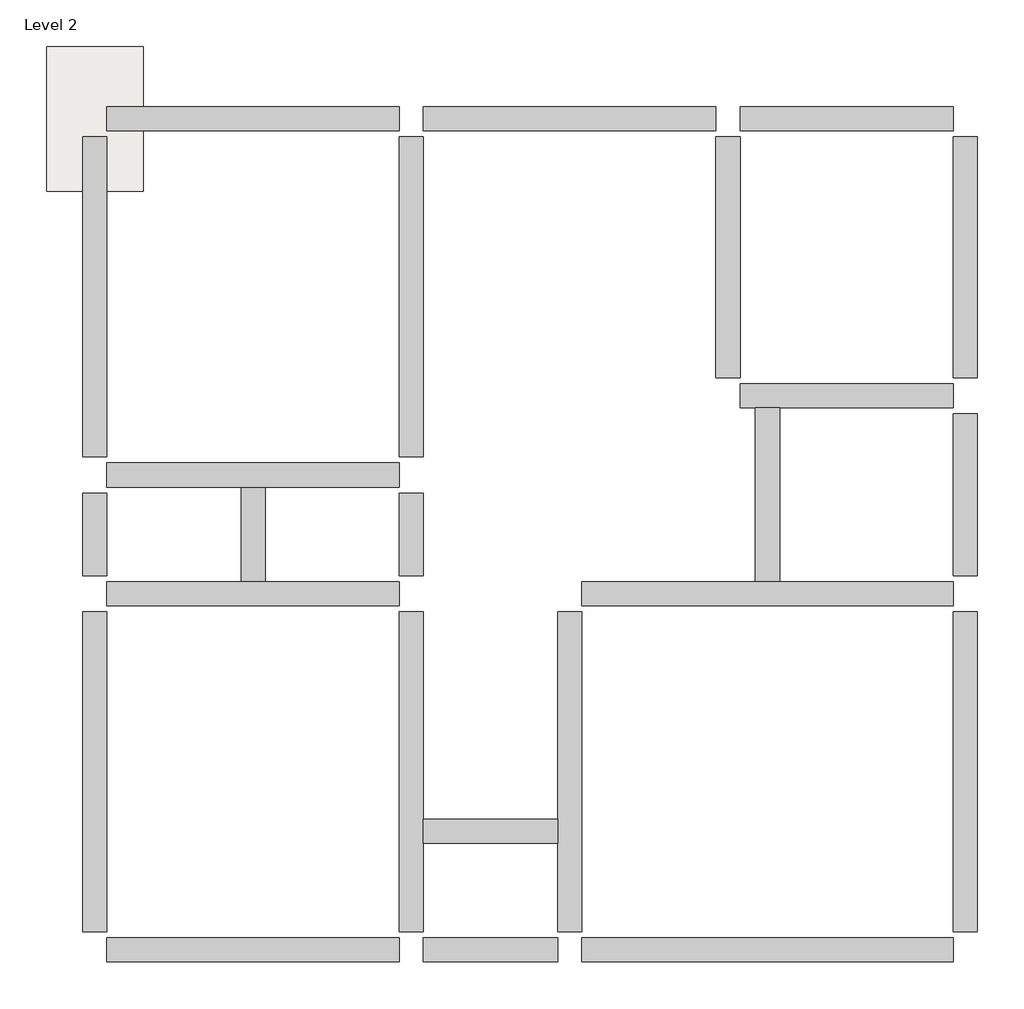
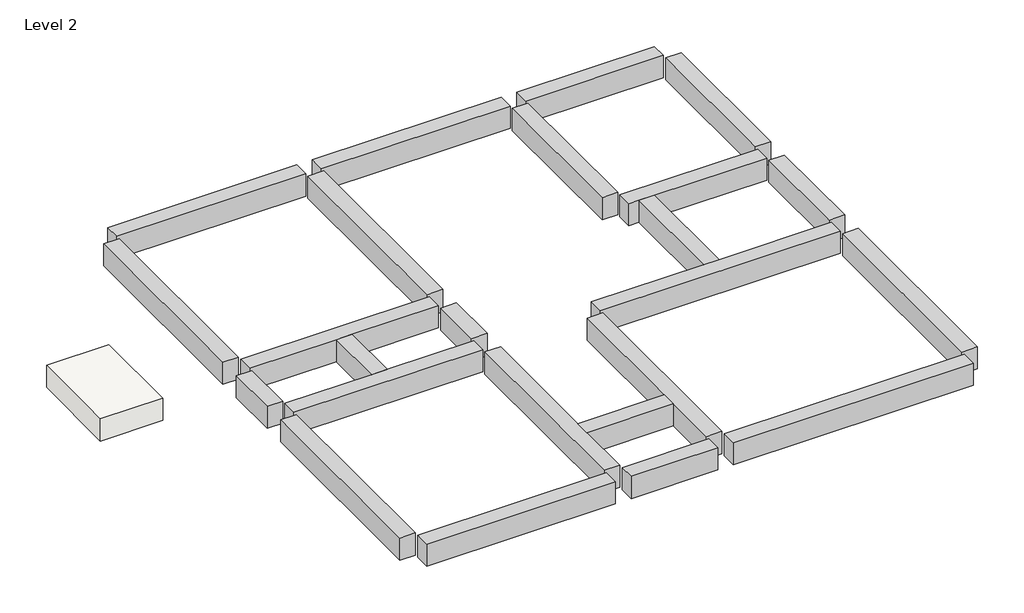
# One storey, part 1 of 5: 14 beams, 1 slab.
"""IFC4 building model written with IfcOpenShell, lengths in millimetres."""

from ifc_helpers import new_model, si_unit, frame, origin, place, context, project, spatial, polyline, outline, extrude, faceted_brep, element, save

model = new_model("IFC4")

# Units and contexts
model_context = context("Model", 3, world=origin())
ifc_project = project(units=[si_unit("LENGTHUNIT", "METRE", prefix="MILLI")], contexts=[model_context])

# Site, building, storey
site = spatial("IfcSite", under=ifc_project)
building = spatial("IfcBuilding", under=site)
storey = spatial("IfcBuildingStorey", under=building, Name="Level 2", Elevation=3048.0)

# Beams
placement = place(None, origin())
element("IfcBeam", 1, ObjectType="Concrete-Rectangular Beam : 12 x 24", at=placement, inside=storey, context=model_context, shape_type="SweptSolid", body=[
    extrude(outline(polyline([(-4459.6215379, 8530.2267522), (-4459.6215379, 8225.4267522), (-7154.8215379, 8225.4267522), (-7154.8215379, 8530.2267522), (-4459.6215379, 8530.2267522)])), frame((0.0, 0.0, 2590.8), z_axis=(0.0, 0.0, 1.0), x_axis=(1.0, 0.0, 0.0)), (0.0, 0.0, 1.0), 457.2),
    extrude(outline(polyline([(-15154.8215379, 8225.4267522), (-15154.8215379, 8530.2267522), (-11459.6215379, 8530.2267522), (-11459.6215379, 8225.4267522), (-15154.8215379, 8225.4267522)])), frame((0.0, 0.0, 2590.8), z_axis=(0.0, 0.0, 1.0), x_axis=(1.0, 0.0, 0.0)), (0.0, 0.0, 1.0), 457.2),
    extrude(outline(polyline([(-11154.8215379, 8225.4267522), (-11154.8215379, 8530.2267522), (-7459.6215379, 8530.2267522), (-7459.6215379, 8225.4267522), (-11154.8215379, 8225.4267522)])), frame((0.0, 0.0, 2590.8), z_axis=(0.0, 0.0, 1.0), x_axis=(1.0, 0.0, 0.0)), (0.0, 0.0, 1.0), 457.2),
])
element("IfcBeam", 2, ObjectType="Concrete-Rectangular Beam : 12 x 24", at=placement, inside=storey, context=model_context, shape_type="SweptSolid", body=[
    extrude(outline(polyline([(-4154.8215379, -1893.5732478), (-4459.6215379, -1893.5732478), (-4459.6215379, 2149.2267522), (-4154.8215379, 2149.2267522), (-4154.8215379, -1893.5732478)])), frame((0.0, 0.0, 2590.8), z_axis=(0.0, 0.0, 1.0), x_axis=(1.0, 0.0, 0.0)), (0.0, 0.0, 1.0), 457.2),
    extrude(outline(polyline([(-4459.6215379, 8149.2267522), (-4154.8215379, 8149.2267522), (-4154.8215379, 5106.4267522), (-4459.6215379, 5106.4267522), (-4459.6215379, 8149.2267522)])), frame((0.0, 0.0, 2590.8), z_axis=(0.0, 0.0, 1.0), x_axis=(1.0, 0.0, 0.0)), (0.0, 0.0, 1.0), 457.2),
    extrude(outline(polyline([(-4154.8215379, 2606.4267522), (-4459.6215379, 2606.4267522), (-4459.6215379, 4649.2267522), (-4154.8215379, 4649.2267522), (-4154.8215379, 2606.4267522)])), frame((0.0, 0.0, 2590.8), z_axis=(0.0, 0.0, 1.0), x_axis=(1.0, 0.0, 0.0)), (0.0, 0.0, 1.0), 457.2),
])
element("IfcBeam", 3, ObjectType="Concrete-Rectangular Beam : 12 x 24", at=placement, inside=storey, context=model_context, shape_type="SweptSolid", body=[
    extrude(outline(polyline([(-15154.8215379, -2274.5732478), (-15154.8215379, -1969.7732478), (-11459.6215379, -1969.7732478), (-11459.6215379, -2274.5732478), (-15154.8215379, -2274.5732478)])), frame((0.0, 0.0, 2590.8), z_axis=(0.0, 0.0, 1.0), x_axis=(1.0, 0.0, 0.0)), (0.0, 0.0, 1.0), 457.2),
    extrude(outline(polyline([(-4459.6215379, -1969.7732478), (-4459.6215379, -2274.5732478), (-9154.8215379, -2274.5732478), (-9154.8215379, -1969.7732478), (-4459.6215379, -1969.7732478)])), frame((0.0, 0.0, 2590.8), z_axis=(0.0, 0.0, 1.0), x_axis=(1.0, 0.0, 0.0)), (0.0, 0.0, 1.0), 457.2),
    extrude(outline(polyline([(-11154.8215379, -2274.5732478), (-11154.8215379, -1969.7732478), (-9459.6215379, -1969.7732478), (-9459.6215379, -2274.5732478), (-11154.8215379, -2274.5732478)])), frame((0.0, 0.0, 2590.8), z_axis=(0.0, 0.0, 1.0), x_axis=(1.0, 0.0, 0.0)), (0.0, 0.0, 1.0), 457.2),
])
element("IfcBeam", 4, ObjectType="Concrete-Rectangular Beam : 12 x 24", at=placement, inside=storey, context=model_context, shape_type="SweptSolid", body=[
    extrude(outline(polyline([(-15459.6215379, 8149.2267522), (-15154.8215379, 8149.2267522), (-15154.8215379, 4106.4267522), (-15459.6215379, 4106.4267522), (-15459.6215379, 8149.2267522)])), frame((0.0, 0.0, 2590.8), z_axis=(0.0, 0.0, 1.0), x_axis=(1.0, 0.0, 0.0)), (0.0, 0.0, 1.0), 457.2),
    extrude(outline(polyline([(-15154.8215379, -1893.5732478), (-15459.6215379, -1893.5732478), (-15459.6215379, 2149.2267522), (-15154.8215379, 2149.2267522), (-15154.8215379, -1893.5732478)])), frame((0.0, 0.0, 2590.8), z_axis=(0.0, 0.0, 1.0), x_axis=(1.0, 0.0, 0.0)), (0.0, 0.0, 1.0), 457.2),
    extrude(outline(polyline([(-15459.6215379, 3649.2267522), (-15154.8215379, 3649.2267522), (-15154.8215379, 2606.4267522), (-15459.6215379, 2606.4267522), (-15459.6215379, 3649.2267522)])), frame((0.0, 0.0, 2590.8), z_axis=(0.0, 0.0, 1.0), x_axis=(1.0, 0.0, 0.0)), (0.0, 0.0, 1.0), 457.2),
])
element("IfcBeam", 5, ObjectType="Concrete-Rectangular Beam : 12 x 24", at=placement, inside=storey, context=model_context, shape_type="Brep", body=[
    faceted_brep([(-11459.6215379, -1893.5732478, 3048.0), (-11154.8215379, -1893.5732478, 3048.0), (-11154.8215379, -774.5732478, 3048.0), (-11154.8215379, -469.7732478, 3048.0), (-11154.8215379, 2149.2267522, 3048.0), (-11459.6215379, 2149.2267522, 3048.0), (-11459.6215379, -1893.5732478, 2590.8), (-11459.6215379, 2149.2267522, 2590.8), (-11154.8215379, -1893.5732478, 2590.8), (-11154.8215379, 2149.2267522, 2590.8), (-11154.8215379, -469.7732478, 2590.8), (-11154.8215379, -774.5732478, 2590.8)], [[[0, 1, 2, 3, 4, 5]], [[6, 0, 5, 7]], [[8, 6, 7, 9, 10, 11]], [[1, 8, 11, 10, 9, 4, 3, 2]], [[1, 0, 6, 8]], [[5, 4, 9, 7]]]),
    faceted_brep([(-11459.6215379, 8149.2267522, 3048.0), (-11154.8215379, 8149.2267522, 3048.0), (-11154.8215379, 8149.2267522, 2590.8), (-11459.6215379, 8149.2267522, 2590.8), (-11154.8215379, 4106.4267522, 3048.0), (-11459.6215379, 4106.4267522, 3048.0), (-11459.6215379, 4106.4267522, 2590.8), (-11154.8215379, 4106.4267522, 2590.8)], [[[0, 1, 2, 3]], [[4, 5, 6, 7]], [[1, 0, 5, 4]], [[0, 3, 6, 5]], [[3, 2, 7, 6]], [[2, 1, 4, 7]]]),
    faceted_brep([(-11459.6215379, 3649.2267522, 3048.0), (-11154.8215379, 3649.2267522, 3048.0), (-11154.8215379, 3649.2267522, 2590.8), (-11459.6215379, 3649.2267522, 2590.8), (-11154.8215379, 2606.4267522, 3048.0), (-11459.6215379, 2606.4267522, 3048.0), (-11459.6215379, 2606.4267522, 2590.8), (-11154.8215379, 2606.4267522, 2590.8)], [[[0, 1, 2, 3]], [[4, 5, 6, 7]], [[1, 0, 5, 4]], [[0, 3, 6, 5]], [[3, 2, 7, 6]], [[2, 1, 4, 7]]]),
])
element("IfcBeam", 6, ObjectType="Concrete-Rectangular Beam : 12 x 24", at=placement, inside=storey, context=model_context, shape_type="Brep", body=[
    faceted_brep([(-9459.6215379, -1893.5732478, 3048.0), (-9154.8215379, -1893.5732478, 3048.0), (-9154.8215379, 2149.2267522, 3048.0), (-9459.6215379, 2149.2267522, 3048.0), (-9459.6215379, -469.7732478, 3048.0), (-9459.6215379, -774.5732478, 3048.0), (-9154.8215379, -1893.5732478, 2590.8), (-9154.8215379, 2149.2267522, 2590.8), (-9459.6215379, -1893.5732478, 2590.8), (-9459.6215379, -774.5732478, 2590.8), (-9459.6215379, -469.7732478, 2590.8), (-9459.6215379, 2149.2267522, 2590.8)], [[[0, 1, 2, 3, 4, 5]], [[1, 6, 7, 2]], [[6, 8, 9, 10, 11, 7]], [[8, 0, 5, 4, 3, 11, 10, 9]], [[1, 0, 8, 6]], [[3, 2, 7, 11]]]),
])
element("IfcBeam", 7, ObjectType="Concrete-Rectangular Beam : 12 x 24", at=placement, inside=storey, context=model_context, shape_type="Brep", body=[
    faceted_brep([(-4459.6215379, 2225.4267522, 3048.0), (-4459.6215379, 2530.2267522, 3048.0), (-6654.8215379, 2530.2267522, 3048.0), (-6959.6215379, 2530.2267522, 3048.0), (-9154.8215379, 2530.2267522, 3048.0), (-9154.8215379, 2225.4267522, 3048.0), (-4459.6215379, 2225.4267522, 2590.8), (-9154.8215379, 2225.4267522, 2590.8), (-4459.6215379, 2530.2267522, 2590.8), (-9154.8215379, 2530.2267522, 2590.8), (-6959.6215379, 2530.2267522, 2590.8), (-6654.8215379, 2530.2267522, 2590.8)], [[[0, 1, 2, 3, 4, 5]], [[6, 0, 5, 7]], [[8, 6, 7, 9, 10, 11]], [[1, 8, 11, 10, 9, 4, 3, 2]], [[1, 0, 6, 8]], [[4, 9, 7, 5]]]),
])
element("IfcBeam", 8, ObjectType="Concrete-Rectangular Beam : 12 x 24", at=placement, inside=storey, context=model_context, shape_type="SweptSolid", body=[
    extrude(outline(polyline([(-7459.6215379, 8149.2267522), (-7154.8215379, 8149.2267522), (-7154.8215379, 5106.4267522), (-7459.6215379, 5106.4267522), (-7459.6215379, 8149.2267522)])), frame((0.0, 0.0, 2590.8), z_axis=(0.0, 0.0, 1.0), x_axis=(1.0, 0.0, 0.0)), (0.0, 0.0, 1.0), 457.2),
])
element("IfcBeam", 9, ObjectType="Concrete-Rectangular Beam : 12 x 24", at=placement, inside=storey, context=model_context, shape_type="Brep", body=[
    faceted_brep([(-7154.8215379, 5030.2267522, 3048.0), (-7154.8215379, 4725.4267522, 3048.0), (-6959.6215379, 4725.4267522, 3048.0), (-6654.8215379, 4725.4267522, 3048.0), (-4459.6215379, 4725.4267522, 3048.0), (-4459.6215379, 5030.2267522, 3048.0), (-7154.8215379, 5030.2267522, 2590.8), (-4459.6215379, 5030.2267522, 2590.8), (-7154.8215379, 4725.4267522, 2590.8), (-4459.6215379, 4725.4267522, 2590.8), (-6654.8215379, 4725.4267522, 2590.8), (-6959.6215379, 4725.4267522, 2590.8)], [[[0, 1, 2, 3, 4, 5]], [[6, 0, 5, 7]], [[8, 6, 7, 9, 10, 11]], [[1, 8, 11, 10, 9, 4, 3, 2]], [[0, 6, 8, 1]], [[5, 4, 9, 7]]]),
])
element("IfcBeam", 10, ObjectType="Concrete-Rectangular Beam : 12 x 24", at=placement, inside=storey, context=model_context, shape_type="Brep", body=[
    faceted_brep([(-15154.8215379, 4030.2267522, 3048.0), (-15154.8215379, 3725.4267522, 3048.0), (-13459.6215379, 3725.4267522, 3048.0), (-13154.8215379, 3725.4267522, 3048.0), (-11459.6215379, 3725.4267522, 3048.0), (-11459.6215379, 4030.2267522, 3048.0), (-15154.8215379, 3725.4267522, 2590.8), (-13459.6215379, 3725.4267522, 2590.8), (-13154.8215379, 3725.4267522, 2590.8), (-11459.6215379, 3725.4267522, 2590.8), (-15154.8215379, 4030.2267522, 2590.8), (-11459.6215379, 4030.2267522, 2590.8)], [[[0, 1, 2, 3, 4, 5]], [[1, 6, 7, 8, 9, 4, 3, 2]], [[6, 10, 11, 9, 8, 7]], [[10, 0, 5, 11]], [[1, 0, 10, 6]], [[5, 4, 9, 11]]]),
])
element("IfcBeam", 11, ObjectType="Concrete-Rectangular Beam : 12 x 24", at=placement, inside=storey, context=model_context, shape_type="Brep", body=[
    faceted_brep([(-15154.8215379, 2530.2267522, 3048.0), (-15154.8215379, 2225.4267522, 3048.0), (-11459.6215379, 2225.4267522, 3048.0), (-11459.6215379, 2530.2267522, 3048.0), (-13154.8215379, 2530.2267522, 3048.0), (-13459.6215379, 2530.2267522, 3048.0), (-15154.8215379, 2530.2267522, 2590.8), (-11459.6215379, 2530.2267522, 2590.8), (-13154.8215379, 2530.2267522, 2590.8), (-13459.6215379, 2530.2267522, 2590.8), (-15154.8215379, 2225.4267522, 2590.8), (-11459.6215379, 2225.4267522, 2590.8)], [[[0, 1, 2, 3, 4, 5]], [[6, 0, 5, 4, 3, 7, 8, 9]], [[10, 6, 9, 8, 7, 11]], [[1, 10, 11, 2]], [[1, 0, 6, 10]], [[3, 2, 11, 7]]]),
])
element("IfcBeam", 12, ObjectType="Concrete-Rectangular Beam : 12 x 24", at=placement, inside=storey, context=model_context, shape_type="SweptSolid", body=[
    extrude(outline(polyline([(-13459.6215379, 3725.4267522), (-13154.8215379, 3725.4267522), (-13154.8215379, 2530.2267522), (-13459.6215379, 2530.2267522), (-13459.6215379, 3725.4267522)])), frame((0.0, 0.0, 2590.8), z_axis=(0.0, 0.0, 1.0), x_axis=(1.0, 0.0, 0.0)), (0.0, 0.0, 1.0), 457.2),
])
element("IfcBeam", 13, ObjectType="Concrete-Rectangular Beam : 12 x 24", at=placement, inside=storey, context=model_context, shape_type="SweptSolid", body=[
    extrude(outline(polyline([(-6654.8215379, 2530.2267522), (-6959.6215379, 2530.2267522), (-6959.6215379, 4725.4267522), (-6654.8215379, 4725.4267522), (-6654.8215379, 2530.2267522)])), frame((0.0, 0.0, 2590.8), z_axis=(0.0, 0.0, 1.0), x_axis=(1.0, 0.0, 0.0)), (0.0, 0.0, 1.0), 457.2),
])
element("IfcBeam", 14, ObjectType="Concrete-Rectangular Beam : 12 x 24", at=placement, inside=storey, context=model_context, shape_type="SweptSolid", body=[
    extrude(outline(polyline([(-11154.8215379, -774.5732478), (-11154.8215379, -469.7732478), (-9459.6215379, -469.7732478), (-9459.6215379, -774.5732478), (-11154.8215379, -774.5732478)])), frame((0.0, 0.0, 2590.8), z_axis=(0.0, 0.0, 1.0), x_axis=(1.0, 0.0, 0.0)), (0.0, 0.0, 1.0), 457.2),
])

# Slab
element("IfcSlab", 15, ObjectType="Footing-Rectangular : 72\" x 48\" x 18\"", at=placement, inside=storey, context=model_context, shape_type="SweptSolid", body=[
    extrude(outline(polyline([(-14697.6215379, 9292.2267522), (-14697.6215379, 7463.4267522), (-15916.8215379, 7463.4267522), (-15916.8215379, 9292.2267522), (-14697.6215379, 9292.2267522)])), frame((0.0, 0.0, -457.2), z_axis=(0.0, 0.0, 1.0), x_axis=(1.0, 0.0, 0.0)), (0.0, 0.0, 1.0), 457.2),
])

save(model, "model.ifc")

# Revit data of these elements
# Type "Concrete-Rectangular Beam : 12 x 24"
#   Assembly Code = "B10"
#   Length [instance default] = 5' - 0"
#   b = 1' - 0"
#   h = 1' - 6"
#   Structural Material [instance default] = Concrete, Cast-in-Place gray
# Type "Footing-Rectangular : 72\" x 48\" x 18\""
#   Assembly Code = "A1010100"
#   Width = 4' - 0"
#   Length = 6' - 0"
#   Foundation Thickness = 1' - 6"
#   Structural Material [instance default] = Concrete, Cast-in-Place gray
# Elements 1, 2, 3, 4, 5, 6, 7, 8, 9, 10, 11, 12, 13, 14 (IfcBeam, "Concrete-Rectangular Beam : 12 x 24")
#   Structural Material = Concrete, Cast-in-Place gray
#   Phase Created = New Construction
#   Materials on its faces: "Concrete, Cast-in-Place gray"
# Element 15 (IfcSlab, "Footing-Rectangular : 72\" x 48\" x 18\"")
#   Structural Material = Concrete, Cast-in-Place gray
#   Phase Created = New Construction
#   Materials on its faces: "Concrete, Cast-in-Place gray"
# Materials
#   "Concrete, Cast-in-Place gray": class "Concrete", colour RGB 192 192 192, transparency 0, Description = "Cast-in-place concrete", Cost = 0
